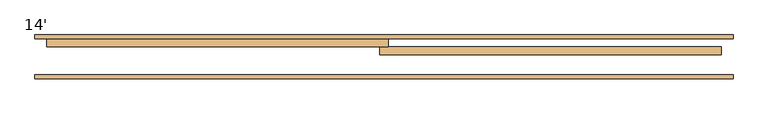
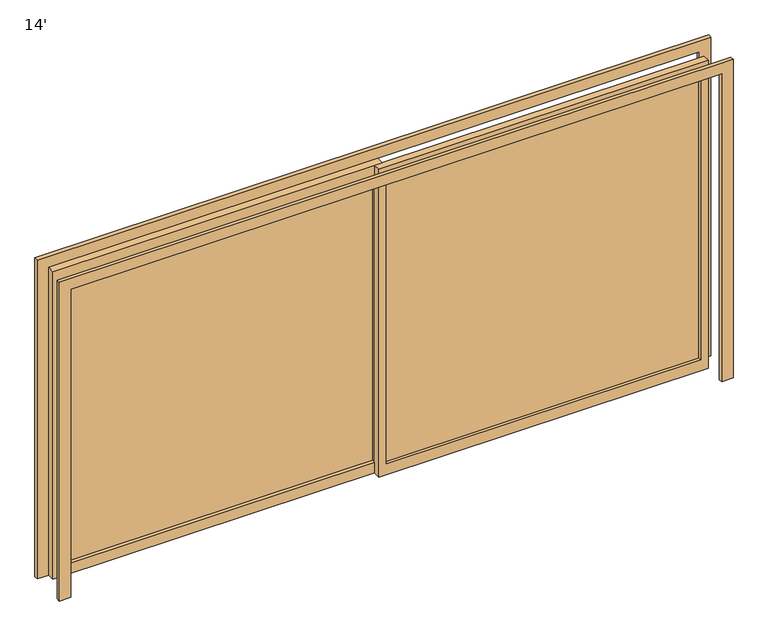
"""IFC4 building model written with IfcOpenShell, lengths in millimetres: door geometry, 14'."""

from ifc_helpers import new_model, si_unit, frame, origin, place, context, project, spatial, polyline, outline, extrude, source, transform, mapped, element, save


def door_14_4c4e9c4f(model_context):
    return source(origin(), model_context, "Body", "SweptSolid", [
        extrude(outline(polyline([(0.0, 2208.6), (2209.0, 2208.6), (2209.0, -2208.6), (0.0, -2208.6), (0.0, -2133.6), (2134.0, -2133.6), (2134.0, 2133.6), (0.0, 2133.6), (0.0, 2208.6)])), frame((0.0, 241.3, 0.0), z_axis=(0.0, 1.0, 0.0), x_axis=(0.0, 0.0, 1.0)), (0.0, 0.0, 1.0), 25.0),
        extrude(outline(polyline([(0.0, -2208.6), (0.0, -2133.6), (2134.0, -2133.6), (2134.0, 2133.6), (0.0, 2133.6), (0.0, 2208.6), (2209.0, 2208.6), (2209.0, -2208.6), (0.0, -2208.6)])), frame((0.0, -12.3, 0.0), z_axis=(0.0, 1.0, 0.0), x_axis=(0.0, 0.0, 1.0)), (0.0, 0.0, 1.0), 25.0),
        extrude(outline(polyline([(2134.0, 25.4), (2134.0, -2133.6), (0.0, -2133.6), (0.0, 25.4), (2134.0, 25.4)]), holes=[polyline([(2059.0, -24.6), (75.0, -24.6), (75.0, -2083.6), (2059.0, -2083.6), (2059.0, -24.6)])]), frame((0.0, 191.3, 0.0), z_axis=(0.0, 1.0, 0.0), x_axis=(0.0, 0.0, 1.0)), (0.0, 0.0, 1.0), 50.0),
        extrude(outline(polyline([(-2083.6, 219.475), (-24.6, 219.475), (-24.6, 213.125), (-2083.6, 213.125), (-2083.6, 219.475)])), frame((0.0, 0.0, 75.0), z_axis=(0.0, 0.0, 1.0), x_axis=(1.0, 0.0, 0.0)), (0.0, 0.0, 1.0), 1984.0),
        extrude(outline(polyline([(2134.0, -25.4), (0.0, -25.4), (0.0, 2133.6), (2134.0, 2133.6), (2134.0, -25.4)]), holes=[polyline([(2059.0, 24.6), (2059.0, 2083.6), (75.0, 2083.6), (75.0, 24.6), (2059.0, 24.6)])]), frame((0.0, 141.3, 0.0), z_axis=(0.0, 1.0, 0.0), x_axis=(0.0, 0.0, 1.0)), (0.0, 0.0, 1.0), 50.0),
        extrude(outline(polyline([(25.4, 169.475), (2083.6, 169.475), (2083.6, 163.125), (25.4, 163.125), (25.4, 169.475)])), frame((0.0, 0.0, 75.0), z_axis=(0.0, 0.0, 1.0), x_axis=(1.0, 0.0, 0.0)), (0.0, 0.0, 1.0), 1984.0),
    ])


if __name__ == "__main__":
    model = new_model("IFC4")
    model_context = context("Model", 3, world=origin())
    ifc_project = project(units=[si_unit("LENGTHUNIT", "METRE", prefix="MILLI")], contexts=[model_context])
    site = spatial("IfcSite", under=ifc_project)
    building = spatial("IfcBuilding", under=site)
    placement = place(None, origin())
    door_14_shape = door_14_4c4e9c4f(model_context)
    element("IfcDoor", 1, ObjectType="14'", at=placement, inside=building, context=model_context, shape_type="MappedRepresentation", body=[
        mapped(door_14_shape, transform((0.0, 0.0, 0.0), x_axis=(1.0, 0.0, 0.0), y_axis=(0.0, 1.0, 0.0), z_axis=(0.0, 0.0, 1.0))),
    ])
    save(model, "model.ifc")

# Revit data of these elements
# Type "14'"
#   Type Mark = "59"
#   Thickness = 0' - 1.9685"
#   Height = 7' - 0.01575"
#   Anchura de barandal = 0' - 2.95276"
#   Anchura de montante = 0' - 1.9685"
#   Proyección cubrejuntas ext. = 0' - 0.98425"
#   Proyección cubrejuntas int. = 0' - 0.98425"
#   Anchura de cubrejuntas = 0' - 2.95276"
#   Width = 14' - 0"
#   Material de puerta = Puerta - Panel
#   Function = (empty or 0)
#   Assembly Code = ""
#   Wall Closure = (empty or 0)
# Element 1 (IfcDoor, "14'")
#   Materials on its faces: "Puerta - Panel", "Cristal"
# Materials
#   "Puerta - Panel": class "Madera", colour RGB 210 159 95, transparency 0
#   "Cristal": class "Vidrio", colour RGB 0 0 255, transparency 0.75
